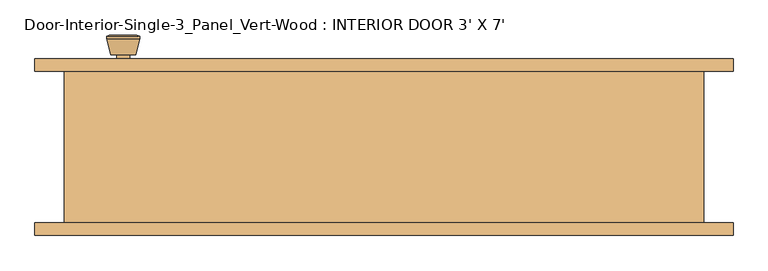
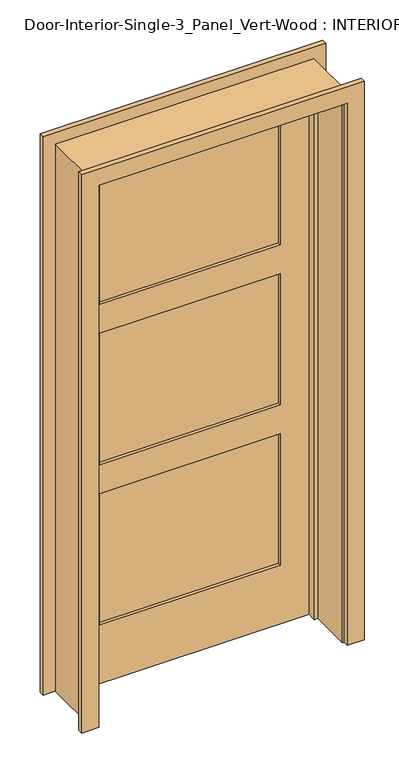
"""IFC4 building model written with IfcOpenShell, lengths in millimetres: door geometry, Door-Interior-Single-3_Panel_Vert-Wood : INTERIOR DOOR 3' X 7'."""

from ifc_helpers import new_model, si_unit, point, frame, frame_2d, origin, place, context, project, spatial, polyline, circle_curve, trimmed, segment, composite_curve, outline, extrude, faceted_brep, source, transform, mapped, element, save
from ifc_brep_helpers import plane_surface, cylinder_surface, revolved_surface, advanced_brep


def door_interior_single_3_panel_vert_wood_interior_door_3_x_7_9905b5e2(model_context):
    return source(origin(), model_context, "Body", "SolidModel", [
        advanced_brep(
        [(-393.7, 70.2, 914.4), (-383.7, 70.2, 914.4), (-403.7, 70.2, 914.4), (-373.2241324, 21.2, 914.4), (-393.7, 21.2, 914.4), (-414.1758676, 21.2, 914.4), (-368.7, 23.0278681, 914.4), (-418.7, 23.0278681, 914.4), (-368.7, 26.4915463, 914.4), (-418.7, 26.4915463, 914.4), (-375.063764, 51.2, 914.4), (-412.336236, 51.2, 914.4), (-383.7, 51.2, 914.4), (-403.7, 51.2, 914.4)],
        [
            (0, 1),
            (1, 2, circle_curve(frame((-393.7, 70.2, 914.4), z_axis=(0.0, 1.0, 0.0), x_axis=(-1.0, 0.0, 0.0)), 10.0)),
            (2, 0),
            (2, 1, circle_curve(frame((-393.7, 70.2, 914.4), z_axis=(0.0, 1.0, 0.0), x_axis=(-1.0, 0.0, 0.0)), 10.0)),
            (3, 4),
            (4, 5),
            (5, 3, circle_curve(frame((-393.7, 21.2, 914.4), z_axis=(0.0, -1.0, 0.0), x_axis=(-1.0, 0.0, 0.0)), 20.4758676)),
            (3, 5, circle_curve(frame((-393.7, 21.2, 914.4), z_axis=(0.0, -1.0, 0.0), x_axis=(-1.0, 0.0, 0.0)), 20.4758676)),
            (6, 3),
            (5, 7),
            (7, 6, circle_curve(frame((-393.7, 23.0278681, 914.4), z_axis=(0.0, -1.0, 0.0), x_axis=(-1.0, 0.0, 0.0)), 25.0)),
            (6, 7, circle_curve(frame((-393.7, 23.0278681, 914.4), z_axis=(0.0, -1.0, 0.0), x_axis=(-1.0, 0.0, 0.0)), 25.0)),
            (8, 6),
            (7, 9),
            (9, 8, circle_curve(frame((-393.7, 26.4915463, 914.4), z_axis=(0.0, -1.0, 0.0), x_axis=(-1.0, 0.0, 0.0)), 25.0)),
            (8, 9, circle_curve(frame((-393.7, 26.4915463, 914.4), z_axis=(0.0, -1.0, 0.0), x_axis=(-1.0, 0.0, 0.0)), 25.0)),
            (10, 8),
            (9, 11),
            (11, 10, circle_curve(frame((-393.7, 51.2, 914.4), z_axis=(0.0, -1.0, 0.0), x_axis=(-1.0, 0.0, 0.0)), 18.636236)),
            (10, 11, circle_curve(frame((-393.7, 51.2, 914.4), z_axis=(0.0, -1.0, 0.0), x_axis=(-1.0, 0.0, 0.0)), 18.636236)),
            (12, 10),
            (11, 13),
            (13, 12, circle_curve(frame((-393.7, 51.2, 914.4), z_axis=(0.0, -1.0, 0.0), x_axis=(-1.0, 0.0, 0.0)), 10.0)),
            (12, 13, circle_curve(frame((-393.7, 51.2, 914.4), z_axis=(0.0, -1.0, 0.0), x_axis=(-1.0, 0.0, 0.0)), 10.0)),
            (1, 12),
            (13, 2),
        ],
        [
            plane_surface(frame((-393.7, 70.2, 914.4), z_axis=(0.0, 1.0, 0.0), x_axis=(-1.0, 0.0, 0.0))),
            plane_surface(frame((-393.7, 21.2, 914.4), z_axis=(0.0, -1.0, 0.0), x_axis=(-1.0, 0.0, 0.0))),
            revolved_surface(polyline([(-414.1758676, 21.2, 914.4), (-418.7, 23.0278681, 914.4)]), (-393.7, 70.2, 914.4), (0.0, 1.0, 0.0)),
            cylinder_surface(frame((-393.7, 70.2, 914.4), z_axis=(0.0, 1.0, 0.0), x_axis=(-1.0, 0.0, 0.0)), 25.0),
            revolved_surface(polyline([(-418.7, 26.4915463, 914.4), (-412.336236, 51.2, 914.4)]), (-393.7, 70.2, 914.4), (0.0, 1.0, 0.0)),
            plane_surface(frame((-393.7, 51.2, 914.4), z_axis=(0.0, 1.0, 0.0), x_axis=(-1.0, 0.0, 0.0))),
            cylinder_surface(frame((-393.7, 70.2, 914.4), z_axis=(0.0, 1.0, 0.0), x_axis=(-1.0, 0.0, 0.0)), 10.0),
        ],
        [
            (0, [[1, 2, 3]]),
            (0, [[-3, 4, -1]]),
            (1, [[5, 6, 7]]),
            (1, [[-6, -5, 8]]),
            (2, [[9, -7, 10, 11]]),
            (2, [[-10, -8, -9, 12]]),
            (3, [[13, -11, 14, 15]]),
            (3, [[-14, -12, -13, 16]]),
            (4, [[17, -15, 18, 19]]),
            (4, [[-18, -16, -17, 20]]),
            (5, [[21, -19, 22, 23]]),
            (5, [[-22, -20, -21, 24]]),
            (6, [[25, -23, 26, -2]]),
            (6, [[-26, -24, -25, -4]]),
        ],
    ),
        extrude(outline(composite_curve([segment(trimmed(circle_curve(frame_2d((914.4, -393.7)), 30.0), [point((914.4, -423.7))], [point((914.4, -363.7))], False, "CARTESIAN"), True, "CONTINUOUS"), segment(trimmed(circle_curve(frame_2d((914.4, -393.7)), 30.0), [point((914.4, -363.7))], [point((914.4, -423.7))], False, "CARTESIAN"), True, "CONTINUOUS")], self_intersect=False)), frame((0.0, 70.2, 0.0), z_axis=(0.0, 1.0, 0.0), x_axis=(0.0, 0.0, 1.0)), (0.0, 0.0, 1.0), 6.0),
        advanced_brep(
        [(-393.7, 117.125, 914.4), (-403.7, 117.125, 914.4), (-383.7, 117.125, 914.4), (-373.2241324, 166.125, 914.4), (-414.1758676, 166.125, 914.4), (-393.7, 166.125, 914.4), (-368.7, 164.2971319, 914.4), (-418.7, 164.2971319, 914.4), (-368.7, 160.8334537, 914.4), (-418.7, 160.8334537, 914.4), (-375.063764, 136.125, 914.4), (-412.336236, 136.125, 914.4), (-383.7, 136.125, 914.4), (-403.7, 136.125, 914.4)],
        [
            (0, 1),
            (1, 2, circle_curve(frame((-393.7, 117.125, 914.4), z_axis=(0.0, -1.0, 0.0), x_axis=(-1.0, 0.0, 0.0)), 10.0)),
            (2, 0),
            (2, 1, circle_curve(frame((-393.7, 117.125, 914.4), z_axis=(0.0, -1.0, 0.0), x_axis=(-1.0, 0.0, 0.0)), 10.0)),
            (3, 4, circle_curve(frame((-393.7, 166.125, 914.4), z_axis=(0.0, 1.0, 0.0), x_axis=(-1.0, 0.0, 0.0)), 20.4758676)),
            (4, 5),
            (5, 3),
            (4, 3, circle_curve(frame((-393.7, 166.125, 914.4), z_axis=(0.0, 1.0, 0.0), x_axis=(-1.0, 0.0, 0.0)), 20.4758676)),
            (6, 7, circle_curve(frame((-393.7, 164.2971319, 914.4), z_axis=(0.0, 1.0, 0.0), x_axis=(-1.0, 0.0, 0.0)), 25.0)),
            (7, 4),
            (3, 6),
            (7, 6, circle_curve(frame((-393.7, 164.2971319, 914.4), z_axis=(0.0, 1.0, 0.0), x_axis=(-1.0, 0.0, 0.0)), 25.0)),
            (8, 9, circle_curve(frame((-393.7, 160.8334537, 914.4), z_axis=(0.0, 1.0, 0.0), x_axis=(-1.0, 0.0, 0.0)), 25.0)),
            (9, 7),
            (6, 8),
            (9, 8, circle_curve(frame((-393.7, 160.8334537, 914.4), z_axis=(0.0, 1.0, 0.0), x_axis=(-1.0, 0.0, 0.0)), 25.0)),
            (10, 11, circle_curve(frame((-393.7, 136.125, 914.4), z_axis=(0.0, 1.0, 0.0), x_axis=(-1.0, 0.0, 0.0)), 18.636236)),
            (11, 9),
            (8, 10),
            (11, 10, circle_curve(frame((-393.7, 136.125, 914.4), z_axis=(0.0, 1.0, 0.0), x_axis=(-1.0, 0.0, 0.0)), 18.636236)),
            (12, 13, circle_curve(frame((-393.7, 136.125, 914.4), z_axis=(0.0, 1.0, 0.0), x_axis=(-1.0, 0.0, 0.0)), 10.0)),
            (13, 11),
            (10, 12),
            (13, 12, circle_curve(frame((-393.7, 136.125, 914.4), z_axis=(0.0, 1.0, 0.0), x_axis=(-1.0, 0.0, 0.0)), 10.0)),
            (1, 13),
            (12, 2),
        ],
        [
            plane_surface(frame((-393.7, 117.125, 914.4), z_axis=(0.0, -1.0, 0.0), x_axis=(-1.0, 0.0, 0.0))),
            plane_surface(frame((-393.7, 166.125, 914.4), z_axis=(0.0, 1.0, 0.0), x_axis=(-1.0, 0.0, 0.0))),
            revolved_surface(polyline([(-414.1758676, 166.125, 914.4), (-418.7, 164.2971319, 914.4)]), (-393.7, 117.125, 914.4), (0.0, -1.0, 0.0)),
            cylinder_surface(frame((-393.7, 117.125, 914.4), z_axis=(0.0, -1.0, 0.0), x_axis=(-1.0, 0.0, 0.0)), 25.0),
            revolved_surface(polyline([(-418.7, 160.8334537, 914.4), (-412.336236, 136.125, 914.4)]), (-393.7, 117.125, 914.4), (0.0, -1.0, 0.0)),
            plane_surface(frame((-393.7, 136.125, 914.4), z_axis=(0.0, -1.0, 0.0), x_axis=(-1.0, 0.0, 0.0))),
            cylinder_surface(frame((-393.7, 117.125, 914.4), z_axis=(0.0, -1.0, 0.0), x_axis=(-1.0, 0.0, 0.0)), 10.0),
        ],
        [
            (0, [[1, 2, 3]]),
            (0, [[-3, 4, -1]]),
            (1, [[5, 6, 7]]),
            (1, [[8, -7, -6]]),
            (2, [[9, 10, -5, 11]]),
            (2, [[12, -11, -8, -10]]),
            (3, [[13, 14, -9, 15]]),
            (3, [[16, -15, -12, -14]]),
            (4, [[17, 18, -13, 19]]),
            (4, [[20, -19, -16, -18]]),
            (5, [[21, 22, -17, 23]]),
            (5, [[24, -23, -20, -22]]),
            (6, [[-2, 25, -21, 26]]),
            (6, [[-4, -26, -24, -25]]),
        ],
    ),
        extrude(outline(composite_curve([segment(trimmed(circle_curve(frame_2d((914.4, -393.7)), 30.0), [point((914.4, -423.7))], [point((914.4, -363.7))], False, "CARTESIAN"), True, "CONTINUOUS"), segment(trimmed(circle_curve(frame_2d((914.4, -393.7)), 30.0), [point((914.4, -363.7))], [point((914.4, -423.7))], False, "CARTESIAN"), True, "CONTINUOUS")], self_intersect=False)), frame((0.0, 111.125, 0.0), z_axis=(0.0, 1.0, 0.0), x_axis=(0.0, 0.0, 1.0)), (0.0, 0.0, 1.0), 6.0),
        faceted_brep([(482.6, 111.125, 0.0), (482.6, -117.475, 0.0), (457.2, -117.475, 0.0), (457.2, 41.275, 0.0), (444.5, 41.275, 0.0), (444.5, 76.2, 0.0), (457.2, 76.2, 0.0), (457.2, 111.125, 0.0), (482.6, 111.125, 2159.0), (482.6, -117.475, 2159.0), (-482.6, -117.475, 2159.0), (-482.6, -117.475, 0.0), (-457.2, -117.475, 0.0), (-457.2, -117.475, 2133.6), (457.2, -117.475, 2133.6), (457.2, 41.275, 2133.6), (-457.2, 41.275, 2133.6), (-457.2, 41.275, 0.0), (-444.5, 41.275, 0.0), (-444.5, 41.275, 2120.9), (444.5, 41.275, 2120.9), (444.5, 76.2, 2120.9), (-444.5, 76.2, 2120.9), (-444.5, 76.2, 0.0), (-457.2, 76.2, 0.0), (-457.2, 76.2, 2133.6), (457.2, 76.2, 2133.6), (457.2, 111.125, 2133.6), (-457.2, 111.125, 2133.6), (-457.2, 111.125, 0.0), (-482.6, 111.125, 0.0), (-482.6, 111.125, 2159.0)], [[[0, 1, 2, 3, 4, 5, 6, 7]], [[1, 0, 8, 9]], [[2, 1, 9, 10, 11, 12, 13, 14]], [[3, 2, 14, 15]], [[4, 3, 15, 16, 17, 18, 19, 20]], [[5, 4, 20, 21]], [[6, 5, 21, 22, 23, 24, 25, 26]], [[7, 6, 26, 27]], [[0, 7, 27, 28, 29, 30, 31, 8]], [[9, 8, 31, 10]], [[15, 14, 13, 16]], [[21, 20, 19, 22]], [[27, 26, 25, 28]], [[30, 29, 24, 23, 18, 17, 12, 11]], [[10, 31, 30, 11]], [[16, 13, 12, 17]], [[22, 19, 18, 23]], [[28, 25, 24, 29]]]),
        extrude(outline(polyline([(2133.6, -457.2), (0.0, -457.2), (0.0, 457.2), (2133.6, 457.2), (2133.6, -457.2)]), holes=[polyline([(2014.5375, -336.55), (2014.5375, 336.55), (1496.4833333, 336.55), (1496.4833333, -336.55), (2014.5375, -336.55)]), polyline([(749.8291667, -336.55), (749.8291667, 336.55), (231.775, 336.55), (231.775, -336.55), (749.8291667, -336.55)]), polyline([(1382.1833333, -336.55), (1382.1833333, 336.55), (864.1291667, 336.55), (864.1291667, -336.55), (1382.1833333, -336.55)])]), frame((0.0, 76.2, 0.0), z_axis=(0.0, 1.0, 0.0), x_axis=(0.0, 0.0, 1.0)), (0.0, 0.0, 1.0), 34.925),
        extrude(outline(polyline([(336.55, 87.8416667), (-336.55, 87.8416667), (-336.55, 99.4833333), (336.55, 99.4833333), (336.55, 87.8416667)])), frame((0.0, 0.0, 1496.4833333), z_axis=(0.0, 0.0, 1.0), x_axis=(1.0, 0.0, 0.0)), (0.0, 0.0, 1.0), 518.0541667),
        extrude(outline(polyline([(336.55, 87.8416667), (-336.55, 87.8416667), (-336.55, 99.4833333), (336.55, 99.4833333), (336.55, 87.8416667)])), frame((0.0, 0.0, 231.775), z_axis=(0.0, 0.0, 1.0), x_axis=(1.0, 0.0, 0.0)), (0.0, 0.0, 1.0), 518.0541667),
        extrude(outline(polyline([(336.55, 87.8416667), (-336.55, 87.8416667), (-336.55, 99.4833333), (336.55, 99.4833333), (336.55, 87.8416667)])), frame((0.0, 0.0, 864.1291667), z_axis=(0.0, 0.0, 1.0), x_axis=(1.0, 0.0, 0.0)), (0.0, 0.0, 1.0), 518.0541667),
        extrude(outline(polyline([(0.0, 463.55), (0.0, 527.05), (2203.45, 527.05), (2203.45, -527.05), (0.0, -527.05), (0.0, -463.55), (2139.95, -463.55), (2139.95, 463.55), (0.0, 463.55)])), frame((0.0, 111.125, 0.0), z_axis=(0.0, 1.0, 0.0), x_axis=(0.0, 0.0, 1.0)), (0.0, 0.0, 1.0), 19.05),
        extrude(outline(polyline([(0.0, 463.55), (0.0, 527.05), (2203.45, 527.05), (2203.45, -527.05), (0.0, -527.05), (0.0, -463.55), (2139.95, -463.55), (2139.95, 463.55), (0.0, 463.55)])), frame((0.0, -136.525, 0.0), z_axis=(0.0, 1.0, 0.0), x_axis=(0.0, 0.0, 1.0)), (0.0, 0.0, 1.0), 19.05),
    ])


if __name__ == "__main__":
    model = new_model("IFC4")
    model_context = context("Model", 3, world=origin())
    ifc_project = project(units=[si_unit("LENGTHUNIT", "METRE", prefix="MILLI")], contexts=[model_context])
    site = spatial("IfcSite", under=ifc_project)
    building = spatial("IfcBuilding", under=site)
    placement = place(None, origin())
    door_interior_single_3_panel_vert_wood_interior_door_3_x_7_shape = door_interior_single_3_panel_vert_wood_interior_door_3_x_7_9905b5e2(model_context)
    element("IfcDoor", 1, ObjectType="Door-Interior-Single-3_Panel_Vert-Wood : INTERIOR DOOR 3' X 7'", at=placement, inside=building, context=model_context, shape_type="MappedRepresentation", body=[
        mapped(door_interior_single_3_panel_vert_wood_interior_door_3_x_7_shape, transform((0.0, 0.0, 0.0), x_axis=(1.0, 0.0, 0.0), y_axis=(0.0, 1.0, 0.0), z_axis=(0.0, 0.0, 1.0))),
    ])
    save(model, "model.ifc")

# Revit data of these elements
# Type "Door-Interior-Single-3_Panel_Vert-Wood : INTERIOR DOOR 3' X 7'"
#   Type Mark = "10"
#   Assembly Code = "C1020300"
#   Analytic Construction = "Wooden"
#   Top Rail = 0' - 4 11/16"
#   Thickness = 0' - 1 3/8"
#   Thermal Resistance (R) = 2.5876 (h·ft²·°F)/BTU
#   Swing Angle [instance default] = 90.00°
#   Stiles = 0' - 4 3/4"
#   Rough Width = 3' - 2"
#   Rough Height = 7' - 1"
#   Intermediate Rail = 0' - 4 1/2"
#   Height = 7' - 0"
#   Width = 3' - 0"
#   Heat Transfer Coefficient (U) = 0.3865 BTU/(h·ft²·°F)
#   Bottom Rail = 0' - 9 1/8"
#   Trim Material = Cherry
#   Panel Material = Cherry
#   Frame Material = Cherry
#   Door Handle Material = Aluminum
#   Visual Light Transmittance = 0
#   Solar Heat Gain Coefficient = 0
#   Wall Closure = (empty or 0)
#   Function = (empty or 0)
# Element 1 (IfcDoor, "Door-Interior-Single-3_Panel_Vert-Wood : INTERIOR DOOR 3' X 7'")
#   Materials on its faces: "Cherry", "Aluminum"
# Materials
#   "Cherry": class "Wood", colour RGB 226 177 128, transparency 0, Description = "Prunus Serotina", Cost = 0
#   "Aluminum": class "Metal", colour RGB 247 247 247, transparency 0, Description = "Aluminum 6061", Cost = 0
